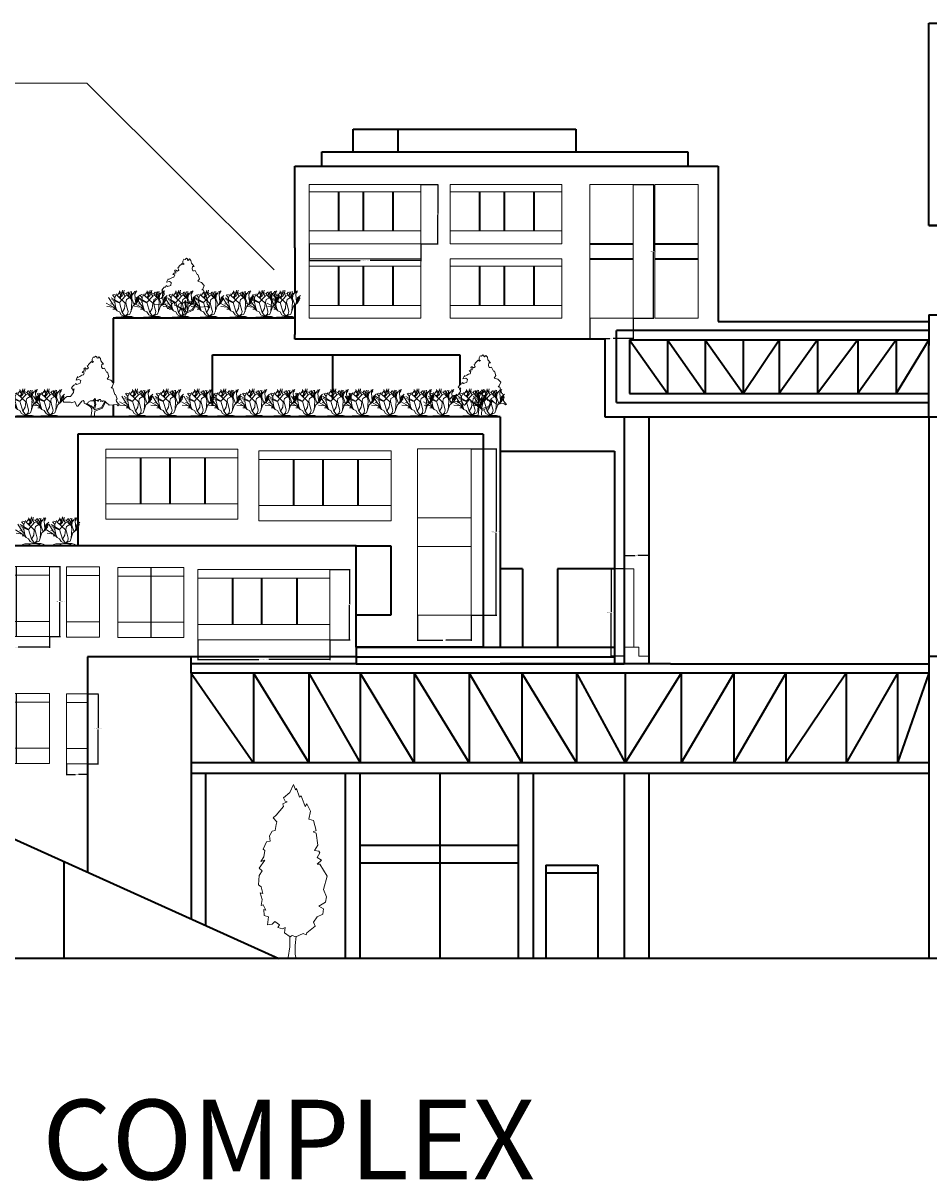
# Model space of a CAD drawing. Units: inches. Extents: x -1080 to 1950, y -1929 to 857.
# Tile 13 of 16: x 294 to 581, y -61 to 305. Entities that reach past the tile are written whole.
import ezdxf

# ---------------------------------------------------------------- set-up
doc = ezdxf.new("R2010")
doc.units = ezdxf.units.IN
doc.header["$MEASUREMENT"] = 0
for name, color, linetype, lineweight in [('A-ANNO-DIMS', 2, 'Continuous', 18), ('A-ANNO-SYMB', 2, 'Continuous', 18), ('A-ANNO-TEXT', 7, 'Continuous', 25), ('A-ELEV', 7, 'Continuous', 35), ('A-GLAZ', 4, 'Continuous', 18), ('L-PLNT', 82, 'Continuous', 13)]:
    doc.layers.add(name, color=color, linetype=linetype, lineweight=lineweight)
doc.styles.get("Standard").update_dxf_attribs({"font": 'arial.ttf'})
doc.dimstyles.get("Standard").update_dxf_attribs({"dimtxt": 0.18, "dimasz": 0.18, "dimexe": 0.18, "dimexo": 0.0625, "dimgap": 0.09, "dimtad": 0, "dimtih": 1, "dimtoh": 1, "dimdec": 4, "dimzin": 0, "dimdsep": 46, "dimtxsty": 'Standard', "dimcen": 0.09, "dimadec": 0, "dimazin": 0, "dimtfac": 1, "dimtdec": 4, "dimtofl": 0, "dimtmove": 0, "dimatfit": 3, "dimfxl": 1, "dimtolj": 1, "dimtzin": 0, "dimarcsym": 0})

# ---------------------------------------------------------------- blocks, each defined once
blk = doc.blocks.new('*U5')
blk.add_lwpolyline([(-2.754, 191.699), (-6.78, 182.851), (-13.682, 176.953), (-11.956, 173.266), (-9.656, 172.529), (-14.257, 170.317), (-13.682, 167.368), (-21.733, 157.783), (-25.184, 154.834), (-21.158, 150.41), (-21.733, 147.461), (-22.884, 140.825), (-26.334, 140.087), (-29.21, 134.926), (-28.635, 129.028), (-32.661, 128.291), (-36.111, 120.18), (-34.386, 118.706), (-35.536, 111.333), (-38.987, 106.171), (-34.386, 107.646), (-40.712, 98.798), (-37.261, 95.849), (-40.712, 90.688), (-41.287, 80.366), (-38.412, 78.154), (-36.686, 70.781), (-39.562, 71.518), (-37.261, 64.145), (-38.412, 57.509), (-36.111, 58.247), (-33.236, 52.348), (-35.536, 53.086), (-34.961, 46.45), (-30.36, 44.975), (-31.51, 36.128), (-26.334, 36.865), (-23.459, 39.814), (-18.283, 36.128), (-20.008, 33.178), (-14.832, 31.704), (-11.956, 33.178), (-12.531, 27.28), (-6.205, 22.856), (-3.905, 24.331), (0.121, 22.856), (8.173, 26.543), (11.624, 25.068), (12.199, 27.28), (21.4, 34.653), (19.675, 39.077), (23.701, 44.975), (30.027, 47.924), (30.602, 53.823), (25.426, 56.772), (32.903, 61.196), (34.053, 67.094), (30.602, 75.205), (34.628, 89.951), (26.576, 103.222), (23.701, 103.222), (28.302, 107.646), (23.701, 110.595), (26.576, 115.756), (25.426, 117.968), (20.825, 118.706), (24.276, 124.604), (22.551, 137.876), (19.1, 139.35), (22.551, 140.825), (19.675, 151.884), (14.499, 153.359), (16.224, 162.207), (12.199, 170.317), (10.473, 167.368), (5.872, 179.165), (4.147, 177.69), (0.696, 187.275), (-0.454, 185.8)], close=True)
for points in [[(-6.813, 23.669), (-6.813, 11.669), (-8.627, 0)], [(0.387, 23.669), (-0.576, 13.271), (-0.576, 3.686), (0, 0)]]:
    blk.add_lwpolyline(points)
blk = doc.blocks.new('*U2')
for points in [[(22.0124, 137.721), (18.5475, 141.5624), (15.5282, 138.2446), (13.8028, 139.3505), (13.3714, 142.1153), (11.2148, 143.2214), (8.1954, 140.4564), (4.7447, 141.0094), (2.1567, 136.0326), (2.1567, 131.6088), (5.6074, 129.9499), (3.0193, 128.2909), (0.4313, 130.5029), (-6.9015, 123.3141), (-6.9015, 121.6552), (-9.9208, 119.9963), (-9.0581, 118.3373), (-6.9015, 115.0195), (-10.7835, 112.2546), (-14.6656, 115.0195), (-16.8222, 114.4665), (-17.6849, 112.2546), (-14.6656, 111.7016), (-14.2342, 107.2778), (-17.6065, 107.8307), (-21.5669, 103.9599), (-17.2536, 103.4069), (-18.9789, 97.8771), (-22.8609, 97.3241), (-27.1743, 94.5593), (-32.3504, 91.7944), (-32.7817, 94.0063), (-36.6638, 85.7116), (-29.7624, 87.3705), (-25.449, 84.6056), (-26.743, 77.9699), (-34.507, 75.205), (-37.9578, 77.4169), (-39.2518, 74.099), (-42.2711, 73.5461), (-44.8592, 70.2282), (-47.8786, 66.3574), (-43.9965, 63.0395), (-41.4085, 64.6985), (-44.3346, 59.8898), (-42.2089, 60.1377), (-42.5159, 55.7849), (-49.6039, 46.4502), (-58.2307, 45.8972), (-62.1127, 43.6853), (-68.5828, 36.4966), (-65.9947, 32.0727), (-50.0352, 32.6257), (-47.0159, 30.4138), (-39.6831, 33.7317), (-34.507, 22.6721), (-32.3504, 22.6721), (-22.4296, 34.8376), (-19.4102, 36.4966), (-17.2536, 33.7317), (-17.2536, 29.8608), (-13.8028, 28.7549), (-9.0581, 28.7549), (-7.3328, 32.6257), (-1.7254, 35.3906), (3.8821, 35.9436), (6.4701, 38.1555), (6.9014, 38.7085), (8.1954, 41.4734), (9.9208, 40.3674), (11.2148, 35.9436), (14.2341, 37.6025), (15.0968, 36.4966), (15.9595, 33.7317), (18.9789, 38.7085), (21.9982, 38.7085), (23.2922, 36.4966), (21.9982, 34.2847), (25.4489, 35.3906), (26.743, 33.7317), (29.7623, 35.9436), (32.7817, 34.8376), (38.8204, 28.7549), (41.4084, 27.6489), (43.5651, 25.437), (61.6813, 27.0959), (65.132, 23.7781), (67.7201, 24.884), (60.8186, 33.7317), (60.3873, 37.0495), (62.544, 40.3674), (58.662, 50.874), (56.5053, 50.874), (52.1919, 66.3574), (47.8785, 66.9103), (50.4665, 69.1222), (53.9172, 77.9699), (47.0158, 85.1586), (38.3891, 87.9235), (42.2711, 94.0063)], [(42.2711, 94.0063), (38.8204, 104.5129), (36.6637, 104.5129), (32.3503, 113.9135), (29.7623, 113.3605), (26.743, 113.3605), (24.5862, 117.7844), (25.8802, 123.8671), (29.331, 123.8671), (22.8609, 131.6088), (21.9982, 137.6916)], [(-12.9401, 28.7549), (-2.588, 22.1191), (0.8626, 17.6953), (1.7253, 11.6125), (0, 0)], [(-9.9208, 28.2019), (0, 23.2251), (3.4507, 19.9072), (4.7447, 15.4834), (8.6267, 27.0959), (6.4701, 37.6025)], [(34.5071, 33.1787), (27.1743, 18.2483), (9.0581, 10.5066), (7.7641, 3.8708), (8.1954, 0)], [(8.1954, 40.3674), (11.2148, 27.6489), (8.1954, 13.8245), (24.5862, 19.9072), (32.7817, 34.2847)]]:
    blk.add_lwpolyline(points)
blk = doc.blocks.new('*U6')
for p, q in [((-377.952, 463.296), (-451.104, 487.68)), ((-426.72, 414.528), (-390.144, 499.872)), ((-377.952, 463.296), (-329.184, 524.256)), ((-316.7634, 502.285), (-327.6092, 559.9176)), ((-296.5958, 484.4034), (-316.7634, 502.285)), ((-286.512, 498.3226), (-307.4416, 538.0736)), ((-302.7934, 478.4344), (-270.256, 518.1854)), ((-290.3982, 464.5406), (-265.6078, 577.8246)), ((-268.7066, 458.5716), (-250.0884, 500.3038)), ((-207.264, 451.104), (-268.224, 548.64)), ((-240.792, 502.285), (-228.3968, 573.8368)), ((-182.88, 499.872), (-219.456, 512.064)), ((-207.264, 451.104), (-134.112, 487.68)), ((-182.88, 499.872), (-158.496, 536.448)), ((-121.92, 414.528), (-182.88, 499.872)), ((-129.1844, 450.6214), (-140.0302, 542.036)), ((-134.112, 487.68), (-97.536, 548.64)), ((-73.152, 329.184), (-109.728, 499.872)), ((-97.536, 426.72), (-24.384, 524.256)), ((-85.7758, 472.4908), (-73.3552, 548.005)), ((-73.152, 402.336), (-60.96, 512.064)), ((-12.9032, 555.9552), (-2.0574, 522.1732)), ((-5.1562, 486.3846), (2.5908, 542.036)), ((8.7884, 335.3562), (-5.1562, 486.3846)), ((-3.6068, 492.3536), (14.986, 518.1854)), ((-0.508, 508.254), (22.7584, 536.067)), ((1.0414, 526.1356), (35.1536, 559.9176)), ((2.5908, 542.036), (21.209, 555.9552)), ((-451.104, 219.456), (-601.0402, 303.8094)), ((-463.296, 280.416), (-552.577, 423.037)), ((-463.296, 280.416), (-512.064, 292.608)), ((-329.184, 316.992), (-499.872, 414.528)), ((-353.568, 316.992), (-487.68, 377.952)), ((-426.72, 414.528), (-475.488, 475.488)), ((-402.336, 207.264), (-463.296, 280.416)), ((-426.72, 316.992), (-451.104, 329.184)), ((-426.72, 316.992), (-426.72, 414.528)), ((-402.336, 207.264), (-426.72, 316.992)), ((-207.264, 304.8), (-377.952, 463.296)), ((-329.184, 316.992), (-353.568, 316.992)), ((-338.455, 424.7896), (-290.3982, 464.5406)), ((-329.184, 316.992), (-207.264, 451.104)), ((-268.224, 109.728), (-329.184, 316.992)), ((-305.8922, 396.9512), (-302.7934, 478.4344)), ((-304.3428, 426.7708), (-268.7066, 458.5716)), ((-219.456, 195.072), (-207.264, 304.8)), ((-195.072, 316.992), (-182.88, 377.952)), ((-170.688, 219.456), (-195.072, 316.992)), ((-182.88, 377.952), (-97.536, 426.72)), ((-85.7758, 389.001), (-129.1844, 452.6026)), ((-109.728, 73.152), (-48.768, 243.84)), ((-70.2564, 426.7708), (-85.7758, 472.4908)), ((-85.344, 134.112), (-73.152, 329.184)), ((-24.384, 268.224), (-73.152, 402.336)), ((-48.768, 243.84), (24.384, 304.8)), ((-12.192, 274.32), (8.7884, 335.3562)), ((8.7884, 335.3562), (33.6042, 412.8516)), ((24.384, 304.8), (36.576, 390.144)), ((24.384, 304.8), (73.152, 377.952)), ((33.6042, 412.8516), (92.5068, 464.5406)), ((36.576, 390.144), (73.152, 438.912)), ((48.768, 341.376), (60.96, 390.144)), ((60.96, 390.144), (85.344, 414.528)), ((-451.104, 219.456), (-587.4512, 234.2388)), ((-414.528, 182.88), (-463.296, 182.88)), ((-377.952, 146.304), (-451.104, 219.456)), ((-402.336, 12.192), (-451.104, 0)), ((-377.952, 146.304), (-402.336, 207.264)), ((-341.376, 12.192), (-402.336, 12.192)), ((-329.184, 121.92), (-377.952, 146.304)), ((-243.84, 24.384), (-341.376, 12.192)), ((-292.608, 60.96), (-329.184, 121.92)), ((-243.84, 24.384), (-329.184, 0)), ((-219.456, 24.384), (-292.608, 60.96)), ((-268.224, 109.728), (-219.456, 195.072)), ((-219.456, 48.768), (-268.224, 109.728)), ((-243.84, 24.384), (-195.072, 24.384)), ((-219.456, 24.384), (-109.728, 73.152)), ((-219.456, 24.384), (-158.496, 73.152)), ((-219.456, 24.384), (-219.456, 48.768)), ((-219.456, 24.384), (-73.152, 24.384)), ((-195.072, 24.384), (-158.496, 12.192)), ((-146.304, 134.112), (-170.688, 219.456)), ((-158.496, 73.152), (-146.304, 134.112)), ((-158.496, 12.192), (-85.344, 0)), ((-73.152, 24.384), (0, 0))]:
    blk.add_line(p, q)
blk = doc.blocks.new('*U4')
for points in [[(559.11496, 3498.1134), (471.1065, 3595.68496), (394.41628, 3511.41284), (350.59112, 3539.5027), (339.63356, 3609.72862), (284.85592, 3637.82356), (208.16316, 3567.59256), (120.51538, 3581.63876), (54.78018, 3455.22804), (54.78018, 3342.86352), (142.42796, 3300.72746), (76.69022, 3258.58886), (10.95502, 3314.77366), (-175.2981, 3132.17814), (-175.2981, 3090.04208), (-251.98832, 3047.90602), (-230.07574, 3005.76742), (-175.2981, 2921.4953), (-273.9009, 2851.26684), (-372.50624, 2921.4953), (-427.28388, 2907.4491), (-449.19646, 2851.26684), (-372.50624, 2837.22064), (-361.54868, 2724.85612), (-447.2051, 2738.89978), (-547.79926, 2640.58146), (-438.24144, 2626.53526), (-482.06406, 2486.07834), (-580.66686, 2472.03214), (-690.22722, 2401.80622), (-821.70016, 2331.57776), (-832.65518, 2387.76002), (-931.26052, 2177.07464), (-755.96496, 2219.2107), (-646.4046, 2148.98224), (-679.2722, 1980.43546), (-876.4778, 1910.207), (-964.12812, 1966.38926), (-996.99572, 1882.1146), (-1073.68594, 1868.07094), (-1139.42368, 1783.79628), (-1216.11644, 1685.47796), (-1117.5111, 1601.2033), (-1051.7759, 1643.3419), (-1126.09884, 1521.20092), (-1072.10606, 1527.49758), (-1079.90386, 1416.93646), (-1259.93906, 1179.83508), (-1479.05978, 1165.78888), (-1577.66258, 1109.60662), (-1742.00312, 927.01364), (-1676.26538, 814.64658), (-1270.89408, 828.69278), (-1194.20386, 772.51052), (-1007.95074, 856.78518), (-876.4778, 575.87134), (-821.70016, 575.87134), (-569.71184, 884.87504), (-493.01908, 927.01364), (-438.24144, 856.78518), (-438.24144, 758.46432), (-350.59112, 730.37446), (-230.07574, 730.37446), (-186.25312, 828.69278), (-43.82516, 898.92124), (98.60534, 912.96744), (164.34054, 969.1497), (175.29556, 983.1959), (208.16316, 1053.42436), (251.98832, 1025.33196), (284.85592, 912.96744), (361.54614, 955.1035), (383.45872, 927.01364), (405.3713, 856.78518), (482.06406, 983.1959), (558.75428, 983.1959), (591.62188, 927.01364), (558.75428, 870.83138), (646.40206, 898.92124), (679.2722, 856.78518), (755.96242, 912.96744), (832.65518, 884.87504), (986.03816, 730.37446), (1051.77336, 702.28206), (1106.55354, 646.0998), (1566.70502, 688.23586), (1654.3528, 603.96374), (1720.09054, 632.0536), (1544.79244, 856.78518), (1533.83742, 941.0573), (1588.6176, 1025.33196), (1490.0148, 1292.1996), (1435.23462, 1292.1996), (1325.67426, 1685.47796), (1216.1139, 1699.52162), (1281.8491, 1755.70388), (1369.49688, 1980.43546), (1194.20132, 2163.02844), (975.08314, 2233.2569), (1073.68594, 2387.76002)], [(1073.68594, 2387.76002), (986.03816, 2654.62766), (931.25798, 2654.62766), (821.69762, 2893.4029), (755.96242, 2879.3567), (679.2722, 2879.3567), (624.48948, 2991.72376), (657.35708, 3146.22434), (745.0074, 3146.22434), (580.66686, 3342.86352), (558.75428, 3497.36664)], [(-328.67854, 730.37446), (-65.7352, 561.82514), (21.91004, 449.46062), (43.82262, 294.9575), (0, 0)], [(-251.98832, 716.32826), (0, 589.91754), (87.64778, 505.64288), (120.51538, 393.27836), (219.11818, 688.23586), (164.34054, 955.1035)], [(876.48034, 842.73898), (690.22722, 463.50682), (230.07574, 266.86764), (197.20814, 98.31832), (208.16316, 0)], [(208.16316, 1025.33196), (284.85592, 702.28206), (208.16316, 351.1423), (624.48948, 505.64288), (832.65518, 870.83138)]]:
    blk.add_lwpolyline(points)
blk = doc.blocks.new('WIN-TYPE-B')
for p, q in [((10.5, 22.21), (0, 22.21)), ((0, 22.21), (0, 19.45)), ((20.91, 22.21), (10.41, 22.21)), ((10.41, 22.21), (10.41, 19.45)), ((10.5, 22.21), (10.5, 19.45)), ((20.91, 22.21), (20.91, 19.45)), ((0, 19.45), (0, 4.84)), ((0, 19.45), (10.5, 19.45)), ((10.41, 19.45), (10.41, 4.84)), ((10.41, 19.45), (20.91, 19.45)), ((10.5, 4.84), (10.5, 19.45)), ((20.91, 4.84), (20.91, 19.45)), ((0, 4.84), (10.5, 4.84)), ((0, 4.84), (0, 0)), ((10.41, 4.84), (20.91, 4.84)), ((10.41, 4.84), (10.41, 0)), ((10.5, 0), (10.5, 4.84)), ((20.91, 0), (20.91, 4.84)), ((0, 0), (10.5, 0)), ((10.41, 0), (20.91, 0))]:
    blk.add_line(p, q)
blk = doc.blocks.new('WIN-TYPE-E')
for p, q in [((10.5, 22.21), (0, 22.21)), ((0, 22.21), (0, 19.45)), ((10.5, 22.21), (10.5, 19.45)), ((0, 19.45), (0, 4.84)), ((0, 19.45), (10.5, 19.45)), ((10.5, 4.84), (10.5, 19.45)), ((0, 4.84), (10.5, 4.84)), ((0, 4.84), (0, 0)), ((10.5, 0), (10.5, 4.84)), ((0, 0), (10.5, 0))]:
    blk.add_line(p, q)
blk = doc.blocks.new('WIN-TYPE-G')
for p, q in [((0, 19.45), (0, 22.21)), ((0, 22.21), (41.85, 22.21)), ((41.85, 22.21), (41.85, 19.45)), ((0, 19.45), (0, 4.84)), ((41.85, 19.45), (0, 19.45)), ((41.85, 4.84), (41.85, 19.45)), ((0, 4.84), (41.85, 4.84)), ((0, 4.84), (0, 0)), ((41.85, 0), (41.85, 4.84)), ((0, 0), (41.85, 0))]:
    blk.add_line(p, q)
blk = doc.blocks.new('WIN-TYPE-H')
for p, q in [((0, 16.47), (0, 18.8)), ((0, 18.8), (35.42, 18.8)), ((35.42, 18.8), (35.42, 16.47)), ((0, 16.47), (0, 4.09)), ((35.42, 16.47), (0, 16.47)), ((35.42, 4.09), (35.42, 16.47)), ((0, 4.09), (35.42, 4.09)), ((0, 4.09), (0, 0)), ((35.42, 0), (35.42, 4.09)), ((0, 0), (35.42, 0))]:
    blk.add_line(p, q)
blk = doc.blocks.new('WIN-TYPE-N')
for p, q in [((0, 52.66), (17.07, 52.66)), ((0, 30.88), (0, 52.66)), ((17.07, 52.66), (17.07, 30.88)), ((17.07, 30.88), (0, 30.88)), ((0, 30.88), (0, 21.78)), ((17.07, 30.88), (17.07, 21.78)), ((0, 21.78), (17.07, 21.78)), ((0, 0), (0, 21.78)), ((17.07, 21.78), (17.07, 0)), ((17.07, 0), (0, 0))]:
    blk.add_line(p, q)
blk = doc.blocks.new('PANEL-A')
for p, q in [((0, 42.42), (0, 0)), ((13.76, 42.42), (0, 42.42)), ((13.76, 0), (13.76, 42.42)), ((0, 0), (13.76, 0))]:
    blk.add_line(p, q)
blk = doc.blocks.new('WIN-TYPE-R')
for p, q in [((6.66, 22.21), (0, 22.21)), ((0, 22.21), (0, 19.45)), ((0, 19.45), (0, 4.84)), ((0, 19.45), (6.66, 19.45)), ((0, 4.84), (6.66, 4.84)), ((0, 4.84), (0, 0)), ((0, 0), (6.66, 0))]:
    blk.add_line(p, q)
blk = doc.blocks.new('WIN-TYPE-S')
for p, q in [((0, 27.66), (3.06, 27.66)), ((3.06, 27.66), (3.06, 2.78)), ((3.06, 2.78), (0, 2.78)), ((3.06, 2.78), (4.6, 2.78)), ((4.6, 2.78), (4.6, 0)), ((4.6, 0), (7.75, 0))]:
    blk.add_line(p, q)
blk = doc.blocks.new('*D37')
at = {"layer": 'A-ANNO-DIMS', "color": 0, "lineweight": -2, "transparency": 16777216}
for p, q in [((302.32, 133.16), (305.76, 133.16)), ((305.58, 132.98), (305.58, 122.24)), ((305.58, 111.13), (305.58, 121.87)), ((302.32, 110.95), (305.76, 110.95))]:
    blk.add_line(p, q, dxfattribs=at)
at = {"layer": 'A-ANNO-DIMS', "color": 0, "transparency": 16777216}
for points in [[(305.55, 132.98), (305.61, 132.98), (305.58, 133.16)], [(305.55, 111.13), (305.61, 111.13), (305.58, 110.95)]]:
    blk.add_solid(points, dxfattribs=at)
at = {"layer": 'Defpoints', "color": 0, "transparency": 16777216}
for p in [(302.25, 133.16), (305.58, 133.16), (302.25, 110.95)]:
    blk.add_point(p, dxfattribs=at)
at = {"layer": 'A-ANNO-DIMS', "color": 0, "transparency": 16777216, "insert": (305.58, 122.05), "char_height": 0.18, "attachment_point": 5}
blk.add_mtext('\\A1;WINDOW TYPE B 22 TYP.', dxfattribs=at)
blk = doc.blocks.new('*D38')
at = {"layer": 'A-ANNO-DIMS', "color": 0, "lineweight": -2, "transparency": 16777216}
for p, q in [((281.34, 110.89), (281.34, 107.44)), ((302.25, 110.89), (302.25, 107.44)), ((281.52, 107.62), (291.27, 107.62)), ((302.07, 107.62), (292.33, 107.62))]:
    blk.add_line(p, q, dxfattribs=at)
at = {"layer": 'A-ANNO-DIMS', "color": 0, "transparency": 16777216}
for points in [[(281.52, 107.65), (281.52, 107.59), (281.34, 107.62)], [(302.07, 107.65), (302.07, 107.59), (302.25, 107.62)]]:
    blk.add_solid(points, dxfattribs=at)
at = {"layer": 'Defpoints', "color": 0, "transparency": 16777216}
for p in [(281.34, 110.95), (302.25, 110.95), (302.25, 107.62)]:
    blk.add_point(p, dxfattribs=at)
at = {"layer": 'A-ANNO-DIMS', "color": 0, "transparency": 16777216, "insert": (291.8, 107.62), "char_height": 0.18, "attachment_point": 5}
blk.add_mtext('\\A1;21 TYP.', dxfattribs=at)
blk = doc.blocks.new('*D47')
at = {"layer": 'A-ANNO-DIMS', "color": 0, "lineweight": -2, "transparency": 16777216}
for p, q in [((349.28, 109.92), (349.28, 103.52)), ((391.12, 109.92), (391.12, 103.52)), ((349.46, 103.7), (368.59, 103.7)), ((390.94, 103.7), (371.82, 103.7))]:
    blk.add_line(p, q, dxfattribs=at)
at = {"layer": 'A-ANNO-DIMS', "color": 0, "transparency": 16777216}
for points in [[(349.46, 103.73), (349.46, 103.67), (349.28, 103.7)], [(390.94, 103.73), (390.94, 103.67), (391.12, 103.7)]]:
    blk.add_solid(points, dxfattribs=at)
at = {"layer": 'Defpoints', "color": 0, "transparency": 16777216}
for p in [(349.28, 109.98), (391.12, 109.98), (391.12, 103.7)]:
    blk.add_point(p, dxfattribs=at)
at = {"layer": 'A-ANNO-DIMS', "color": 0, "transparency": 16777216, "insert": (370.2, 103.7), "char_height": 0.18, "attachment_point": 5}
blk.add_mtext('\\A1;WINDOW TYPE G 42 TYP.', dxfattribs=at)
blk = doc.blocks.new('*D48')
at = {"layer": 'A-ANNO-DIMS', "color": 0, "lineweight": -2, "transparency": 16777216}
for p, q in [((391.19, 132.19), (397.58, 132.19)), ((397.4, 132.01), (397.4, 121.27)), ((397.4, 110.16), (397.4, 120.9)), ((391.19, 109.98), (397.58, 109.98))]:
    blk.add_line(p, q, dxfattribs=at)
at = {"layer": 'A-ANNO-DIMS', "color": 0, "transparency": 16777216}
for points in [[(397.37, 132.01), (397.43, 132.01), (397.4, 132.19)], [(397.37, 110.16), (397.43, 110.16), (397.4, 109.98)]]:
    blk.add_solid(points, dxfattribs=at)
at = {"layer": 'Defpoints', "color": 0, "transparency": 16777216}
for p in [(391.12, 132.19), (397.4, 132.19), (391.12, 109.98)]:
    blk.add_point(p, dxfattribs=at)
at = {"layer": 'A-ANNO-DIMS', "color": 0, "transparency": 16777216, "insert": (397.4, 121.08), "char_height": 0.18, "attachment_point": 5}
blk.add_mtext('\\A1;22 TYP.', dxfattribs=at)
blk = doc.blocks.new('*D49')
at = {"layer": 'A-ANNO-DIMS', "color": 0, "lineweight": -2, "transparency": 16777216}
for p, q in [((384.59, 235.36), (384.59, 229.93)), ((420.01, 235.36), (420.01, 229.93)), ((384.77, 230.11), (400.7, 230.11)), ((419.83, 230.11), (403.91, 230.11))]:
    blk.add_line(p, q, dxfattribs=at)
at = {"layer": 'A-ANNO-DIMS', "color": 0, "transparency": 16777216}
for points in [[(384.77, 230.14), (384.77, 230.08), (384.59, 230.11)], [(419.83, 230.14), (419.83, 230.08), (420.01, 230.11)]]:
    blk.add_solid(points, dxfattribs=at)
at = {"layer": 'Defpoints', "color": 0, "transparency": 16777216}
for p in [(384.59, 235.42), (420.01, 235.42), (420.01, 230.11)]:
    blk.add_point(p, dxfattribs=at)
at = {"layer": 'A-ANNO-DIMS', "color": 0, "transparency": 16777216, "insert": (402.3, 230.11), "char_height": 0.18, "attachment_point": 5}
blk.add_mtext('\\A1;WINDOW TYPE H 35 TYP.', dxfattribs=at)
blk = doc.blocks.new('*D50')
at = {"layer": 'A-ANNO-DIMS', "color": 0, "lineweight": -2, "transparency": 16777216}
for p, q in [((420.08, 254.22), (425.51, 254.22)), ((425.33, 254.04), (425.33, 245)), ((425.33, 235.6), (425.33, 244.64)), ((420.08, 235.42), (425.51, 235.42))]:
    blk.add_line(p, q, dxfattribs=at)
at = {"layer": 'A-ANNO-DIMS', "color": 0, "transparency": 16777216}
for points in [[(425.3, 254.04), (425.36, 254.04), (425.33, 254.22)], [(425.3, 235.6), (425.36, 235.6), (425.33, 235.42)]]:
    blk.add_solid(points, dxfattribs=at)
at = {"layer": 'Defpoints', "color": 0, "transparency": 16777216}
for p in [(420.01, 254.22), (425.33, 254.22), (420.01, 235.42)]:
    blk.add_point(p, dxfattribs=at)
at = {"layer": 'A-ANNO-DIMS', "color": 0, "transparency": 16777216, "insert": (425.33, 244.82), "char_height": 0.18, "attachment_point": 5}
blk.add_mtext('\\A1;19 TYP.', dxfattribs=at)
blk = doc.blocks.new('*D59')
at = {"layer": 'A-ANNO-DIMS', "color": 0, "lineweight": -2, "transparency": 16777216}
for p, q in [((436.01, 170.39), (444.03, 170.39)), ((443.85, 170.21), (443.85, 144.25)), ((443.85, 117.91), (443.85, 143.88)), ((436.01, 117.73), (444.03, 117.73))]:
    blk.add_line(p, q, dxfattribs=at)
at = {"layer": 'A-ANNO-DIMS', "color": 0, "transparency": 16777216}
for points in [[(443.82, 170.21), (443.88, 170.21), (443.85, 170.39)], [(443.82, 117.91), (443.88, 117.91), (443.85, 117.73)]]:
    blk.add_solid(points, dxfattribs=at)
at = {"layer": 'Defpoints', "color": 0, "transparency": 16777216}
for p in [(435.95, 170.39), (443.85, 170.39), (435.95, 117.73)]:
    blk.add_point(p, dxfattribs=at)
at = {"layer": 'A-ANNO-DIMS', "color": 0, "transparency": 16777216, "insert": (443.85, 144.06), "char_height": 0.18, "attachment_point": 5}
blk.add_mtext('\\A1;WINDOW TYPE N 53 TYP.', dxfattribs=at)
blk = doc.blocks.new('*D60')
at = {"layer": 'A-ANNO-DIMS', "color": 0, "lineweight": -2, "transparency": 16777216}
for p, q in [((418.88, 117.67), (418.88, 109.65)), ((435.95, 117.67), (435.95, 109.65)), ((419.06, 109.83), (426.89, 109.83)), ((435.77, 109.83), (427.93, 109.83))]:
    blk.add_line(p, q, dxfattribs=at)
at = {"layer": 'A-ANNO-DIMS', "color": 0, "transparency": 16777216}
for points in [[(419.06, 109.86), (419.06, 109.8), (418.88, 109.83)], [(435.77, 109.86), (435.77, 109.8), (435.95, 109.83)]]:
    blk.add_solid(points, dxfattribs=at)
at = {"layer": 'Defpoints', "color": 0, "transparency": 16777216}
for p in [(418.88, 117.73), (435.95, 117.73), (435.95, 109.83)]:
    blk.add_point(p, dxfattribs=at)
at = {"layer": 'A-ANNO-DIMS', "color": 0, "transparency": 16777216, "insert": (427.41, 109.83), "char_height": 0.18, "attachment_point": 5}
blk.add_mtext('\\A1;17 TYP.', dxfattribs=at)
blk = doc.blocks.new('*D65')
at = {"layer": 'A-ANNO-DIMS', "color": 0, "lineweight": -2, "transparency": 16777216}
for p, q in [((314.38, 92.83), (317.83, 92.83)), ((317.65, 92.65), (317.65, 81.91)), ((317.65, 70.8), (317.65, 81.54)), ((314.38, 70.62), (317.83, 70.62))]:
    blk.add_line(p, q, dxfattribs=at)
at = {"layer": 'A-ANNO-DIMS', "color": 0, "transparency": 16777216}
for points in [[(317.62, 92.65), (317.68, 92.65), (317.65, 92.83)], [(317.62, 70.8), (317.68, 70.8), (317.65, 70.62)]]:
    blk.add_solid(points, dxfattribs=at)
at = {"layer": 'Defpoints', "color": 0, "transparency": 16777216}
for p in [(314.32, 92.83), (317.65, 92.83), (314.32, 70.62)]:
    blk.add_point(p, dxfattribs=at)
at = {"layer": 'A-ANNO-DIMS', "color": 0, "transparency": 16777216, "insert": (317.65, 81.73), "char_height": 0.18, "attachment_point": 5}
blk.add_mtext('\\A1;WINDOW TYPE R 22 TYP.', dxfattribs=at)
blk = doc.blocks.new('*D66')
at = {"layer": 'A-ANNO-DIMS', "color": 0, "lineweight": -2, "transparency": 16777216}
for p, q in [((307.66, 70.56), (307.66, 67.11)), ((314.32, 70.56), (314.32, 67.11)), ((307.84, 67.29), (310.53, 67.29)), ((314.14, 67.29), (311.45, 67.29))]:
    blk.add_line(p, q, dxfattribs=at)
at = {"layer": 'A-ANNO-DIMS', "color": 0, "transparency": 16777216}
for points in [[(307.84, 67.32), (307.84, 67.26), (307.66, 67.29)], [(314.14, 67.32), (314.14, 67.26), (314.32, 67.29)]]:
    blk.add_solid(points, dxfattribs=at)
at = {"layer": 'Defpoints', "color": 0, "transparency": 16777216}
for p in [(307.66, 70.62), (314.32, 70.62), (314.32, 67.29)]:
    blk.add_point(p, dxfattribs=at)
at = {"layer": 'A-ANNO-DIMS', "color": 0, "transparency": 16777216, "insert": (310.99, 67.29), "char_height": 0.18, "attachment_point": 5}
blk.add_mtext('\\A1;7 TYP.', dxfattribs=at)
blk = doc.blocks.new('*D67')
at = {"layer": 'A-ANNO-DIMS', "color": 0, "lineweight": -2, "transparency": 16777216}
for p, q in [((484.36, 132.47), (480.1, 132.47)), ((480.28, 132.29), (480.28, 118.82)), ((480.28, 104.99), (480.28, 118.45)), ((484.36, 104.81), (480.1, 104.81))]:
    blk.add_line(p, q, dxfattribs=at)
at = {"layer": 'A-ANNO-DIMS', "color": 0, "transparency": 16777216}
for points in [[(480.25, 132.29), (480.31, 132.29), (480.28, 132.47)], [(480.25, 104.99), (480.31, 104.99), (480.28, 104.81)]]:
    blk.add_solid(points, dxfattribs=at)
at = {"layer": 'Defpoints', "color": 0, "transparency": 16777216}
for p in [(480.28, 132.47), (484.43, 132.47), (484.43, 104.81)]:
    blk.add_point(p, dxfattribs=at)
at = {"layer": 'A-ANNO-DIMS', "color": 0, "transparency": 16777216, "insert": (480.28, 118.64), "char_height": 0.18, "attachment_point": 5}
blk.add_mtext('\\A1;WINDOW TYPE S 28 TYP.', dxfattribs=at)
blk = doc.blocks.new('*D68')
at = {"layer": 'A-ANNO-DIMS', "color": 0, "lineweight": -2, "transparency": 16777216}
for p, q in [((484.43, 132.53), (484.43, 136.79)), ((484.61, 136.61), (487.85, 136.61)), ((492, 136.61), (488.76, 136.61)), ((492.18, 132.53), (492.18, 136.79))]:
    blk.add_line(p, q, dxfattribs=at)
at = {"layer": 'A-ANNO-DIMS', "color": 0, "transparency": 16777216}
for points in [[(484.61, 136.64), (484.61, 136.58), (484.43, 136.61)], [(492, 136.64), (492, 136.58), (492.18, 136.61)]]:
    blk.add_solid(points, dxfattribs=at)
at = {"layer": 'Defpoints', "color": 0, "transparency": 16777216}
for p in [(492.18, 136.61), (484.43, 132.47), (492.18, 132.47)]:
    blk.add_point(p, dxfattribs=at)
at = {"layer": 'A-ANNO-DIMS', "color": 0, "transparency": 16777216, "insert": (488.3, 136.61), "char_height": 0.18, "attachment_point": 5}
blk.add_mtext('\\A1;8 TYP.', dxfattribs=at)
blk = doc.blocks.new('*D71')
at = {"layer": 'A-ANNO-DIMS', "color": 0, "lineweight": -2, "transparency": 16777216}
for p, q in [((487.36, 254.22), (493.84, 254.22)), ((493.66, 254.04), (493.66, 233.19)), ((493.66, 211.98), (493.66, 232.83)), ((487.36, 211.8), (493.84, 211.8))]:
    blk.add_line(p, q, dxfattribs=at)
at = {"layer": 'A-ANNO-DIMS', "color": 0, "transparency": 16777216}
for points in [[(493.63, 254.04), (493.69, 254.04), (493.66, 254.22)], [(493.63, 211.98), (493.69, 211.98), (493.66, 211.8)]]:
    blk.add_solid(points, dxfattribs=at)
at = {"layer": 'Defpoints', "color": 0, "transparency": 16777216}
for p in [(487.3, 254.22), (493.66, 254.22), (487.3, 211.8)]:
    blk.add_point(p, dxfattribs=at)
at = {"layer": 'A-ANNO-DIMS', "color": 0, "transparency": 16777216, "insert": (493.66, 233.01), "char_height": 0.18, "attachment_point": 5}
blk.add_mtext('\\A1;PANEL A 42 TYP.', dxfattribs=at)
blk = doc.blocks.new('*D72')
at = {"layer": 'A-ANNO-DIMS', "color": 0, "lineweight": -2, "transparency": 16777216}
for p, q in [((473.54, 211.74), (473.54, 205.26)), ((487.3, 211.74), (487.3, 205.26)), ((473.72, 205.44), (479.9, 205.44)), ((487.12, 205.44), (480.94, 205.44))]:
    blk.add_line(p, q, dxfattribs=at)
at = {"layer": 'A-ANNO-DIMS', "color": 0, "transparency": 16777216}
for points in [[(473.72, 205.47), (473.72, 205.41), (473.54, 205.44)], [(487.12, 205.47), (487.12, 205.41), (487.3, 205.44)]]:
    blk.add_solid(points, dxfattribs=at)
at = {"layer": 'Defpoints', "color": 0, "transparency": 16777216}
for p in [(473.54, 211.8), (487.3, 211.8), (487.3, 205.44)]:
    blk.add_point(p, dxfattribs=at)
at = {"layer": 'A-ANNO-DIMS', "color": 0, "transparency": 16777216, "insert": (480.42, 205.44), "char_height": 0.18, "attachment_point": 5}
blk.add_mtext('\\A1;14 TYP.', dxfattribs=at)

msp = doc.modelspace()

# ---------------------------------------------------------------- linework, layer by layer
at = {"layer": 'A-ANNO-SYMB'}
for q in [(282.36, 286.23), (373.52, 227.18)]:
    msp.add_line((314.15, 286.23), q, dxfattribs=at)
at = {"layer": 'A-ELEV'}
for p, q in [((580.98, 305.29), (695.2, 305.29)), ((580.98, 241.18), (580.98, 305.29)), ((398.48, 269.6), (398.48, 271.66)), ((398.48, 271.66), (469.06, 271.66)), ((412.81, 264.54), (412.81, 271.66)), ((469.06, 271.66), (469.06, 264.54)), ((398.48, 264.54), (398.48, 269.6)), ((388.54, 260.04), (388.54, 264.54)), ((388.54, 264.54), (504.61, 264.54)), ((504.61, 264.54), (504.61, 260.04)), ((379.98, 250.46), (379.98, 260.04)), ((379.98, 260.04), (509.7, 260.04)), ((509.7, 260.04), (514.2, 260.04)), ((514.2, 260.04), (514.2, 210.83)), ((379.98, 234.12), (379.98, 250.46)), ((393.87, 251.89), (393.87, 239.51)), ((401.72, 251.89), (401.72, 239.51)), ((411.12, 251.89), (411.12, 239.51)), ((438.56, 251.89), (438.56, 239.51)), ((446.4, 251.89), (446.4, 239.51)), ((455.81, 251.89), (455.81, 239.51)), ((592.18, 241.18), (580.98, 241.18)), ((580.98, 241.18), (695.2, 241.18)), ((473.54, 235.42), (487.3, 235.42)), ((494.09, 235.42), (507.85, 235.42)), ((379.98, 234.12), (379.98, 219.88)), ((393.87, 228.27), (393.87, 215.89)), ((401.72, 228.27), (401.72, 215.89)), ((411.12, 228.27), (411.12, 215.89)), ((438.56, 228.27), (438.56, 215.89)), ((446.4, 228.27), (446.4, 215.89)), ((455.81, 228.27), (455.81, 215.89)), ((473.54, 230.6), (487.3, 230.6)), ((494.09, 230.6), (507.85, 230.6)), ((379.98, 216.14), (379.98, 206.68)), ((580.98, 212.94), (580.98, 203.15)), ((580.98, 212.94), (695.2, 212.94)), ((379.98, 211.8), (322.42, 211.8)), ((322.42, 211.8), (322.42, 191.39)), ((514.2, 210.83), (580.98, 210.83)), ((379.98, 205.21), (379.98, 206.68)), ((580.98, 207.88), (481.95, 207.88)), ((481.95, 185.16), (481.95, 207.88)), ((478.29, 205.21), (379.98, 205.21)), ((478.29, 205.21), (478.29, 185.16)), ((486.15, 204.96), (580.98, 204.96)), ((486.15, 204.96), (486.15, 188.02)), ((486.15, 204.96), (498.15, 188.02)), ((498.15, 204.96), (498.15, 188.02)), ((498.15, 204.96), (510.1, 188.02)), ((510.1, 204.96), (510.1, 188.02)), ((510.1, 204.96), (522.17, 188.02)), ((522.17, 204.96), (522.17, 188.02)), ((522.17, 188.02), (533.52, 204.96)), ((533.52, 204.96), (533.52, 188.02)), ((545.71, 204.96), (533.52, 188.02)), ((545.71, 204.96), (545.71, 188.02)), ((558.5, 204.96), (545.71, 188.02)), ((558.5, 204.96), (558.5, 188.02)), ((570.57, 204.96), (558.5, 188.02)), ((570.57, 204.96), (570.57, 188.02)), ((580.98, 204.96), (570.57, 188.02)), ((580.98, 180.63), (580.98, 203.15)), ((353.96, 187.18), (353.96, 200.27)), ((353.96, 200.27), (432.33, 200.27)), ((391.97, 200.27), (391.97, 186.07)), ((432.33, 200.27), (432.33, 190.71)), ((580.98, 183.28), (580.98, 200.23)), ((486.15, 188.02), (580.98, 188.02)), ((322.42, 184.41), (322.42, 180.63)), ((353.96, 184.1), (353.96, 185.92)), ((478.29, 185.16), (478.29, 180.63)), ((481.95, 185.16), (580.98, 185.16)), ((445.1, 180.63), (264.78, 180.63)), ((391.97, 180.95), (391.97, 180.63)), ((432.51, 180.68), (432.51, 180.63)), ((445.1, 180.63), (445.1, 107.59)), ((478.29, 180.63), (695.2, 180.63)), ((484.43, 180.63), (484.43, 102.28)), ((492.18, 180.63), (492.18, 102.28)), ((580.98, 180.63), (580.98, 104.79)), ((439.77, 175.14), (311.23, 175.14)), ((311.23, 175.14), (311.23, 146.63)), ((439.77, 175.14), (439.77, 107.59)), ((445.1, 169.72), (481.39, 169.72)), ((481.39, 169.72), (481.39, 102.28)), ((331.1, 167.62), (331.1, 153)), ((340.37, 167.62), (340.37, 153)), ((351.48, 167.62), (351.48, 153)), ((379.62, 167.07), (379.62, 152.45)), ((388.89, 167.07), (388.89, 152.45)), ((400, 167.07), (400, 152.45)), ((311.23, 145.47), (311.23, 139.7)), ((311.23, 139.7), (27.33, 139.7)), ((399.5, 139.7), (311.23, 139.7)), ((399.5, 107.59), (399.5, 139.7)), ((399.5, 139.7), (410.5, 139.7)), ((410.5, 139.7), (410.5, 117.73)), ((452.21, 132.47), (445.1, 132.47)), ((452.21, 132.47), (452.21, 107.59)), ((481.39, 132.47), (463.32, 132.47)), ((463.32, 132.47), (463.32, 107.59)), ((360.24, 129.43), (360.24, 114.82)), ((369.51, 129.43), (369.51, 114.82)), ((380.62, 129.43), (380.62, 114.82)), ((410.5, 117.73), (399.5, 117.73)), ((439.77, 107.59), (399.5, 107.59)), ((399.5, 107.59), (399.5, 102.28)), ((399.5, 107.59), (481.39, 107.59)), ((399.5, 104.57), (314.32, 104.57)), ((314.32, 104.57), (314.32, 102.28)), ((347.2, 102.28), (347.2, 104.57)), ((399.5, 104.57), (481.39, 104.57)), ((580.98, 104.79), (695.2, 104.79)), ((580.98, 104.79), (580.98, 65.68)), ((314.32, 102.28), (314.32, 36.38)), ((399.5, 102.28), (347.2, 102.28)), ((347.2, 99.4), (347.2, 102.28)), ((399.5, 99.4), (347.2, 99.4)), ((347.2, 99.4), (347.2, 25.36)), ((347.2, 99.4), (366.88, 70.95)), ((366.88, 99.4), (366.88, 70.95)), ((366.88, 99.4), (384.43, 70.95)), ((384.43, 99.4), (384.43, 70.95)), ((384.43, 99.4), (400.7, 70.95)), ((399.5, 102.28), (484.43, 102.28)), ((495.98, 99.4), (399.5, 99.4)), ((400.7, 99.4), (400.7, 70.95)), ((400.7, 99.4), (417.81, 70.95)), ((417.81, 99.4), (417.81, 70.95)), ((417.81, 99.4), (435.24, 70.95)), ((435.24, 99.4), (435.24, 70.95)), ((435.24, 99.4), (451.98, 70.95)), ((499.06, 102.28), (445.1, 102.28)), ((451.98, 99.4), (451.98, 70.95)), ((451.98, 99.4), (469.32, 70.95)), ((469.32, 99.4), (469.32, 70.95)), ((469.32, 99.4), (484.68, 70.95)), ((484.68, 99.4), (484.68, 70.95)), ((502.48, 99.4), (484.68, 70.95)), ((580.98, 99.4), (495.98, 99.4)), ((499.06, 102.28), (580.98, 102.28)), ((502.48, 99.4), (502.48, 70.95)), ((519.22, 99.4), (502.48, 70.95)), ((519.22, 99.4), (519.22, 70.95)), ((535.61, 99.4), (519.22, 70.95)), ((535.61, 99.4), (535.61, 70.95)), ((554.76, 99.4), (535.61, 70.95)), ((554.76, 99.4), (554.76, 70.95)), ((571.04, 99.4), (554.76, 70.95)), ((571.04, 99.4), (571.04, 70.95)), ((580.98, 99.4), (571.04, 70.95)), ((221.9, 78.07), (374.96, 9.02)), ((499.06, 70.95), (347.2, 70.95)), ((580.98, 70.95), (499.06, 70.95)), ((510.1, 67.56), (347.2, 67.56)), ((351.73, 67.56), (351.73, 19.5)), ((395.95, 67.56), (395.95, 9.02)), ((400.61, 67.56), (400.61, 9.02)), ((426.02, 67.56), (426.02, 9.02)), ((450.86, 67.56), (450.86, 9.02)), ((455.52, 67.56), (455.52, 9.02)), ((484.43, 67.56), (484.43, 9.02)), ((492.18, 67.56), (492.18, 9.02)), ((580.98, 67.56), (510.1, 67.56)), ((580.98, 65.68), (580.98, 9.02)), ((400.61, 44.86), (450.86, 44.86)), ((306.83, 39.76), (306.83, 9.02)), ((400.61, 39.31), (450.86, 39.31)), ((459.6, 38.54), (476.06, 38.54)), ((459.6, 38.54), (459.6, 9.02)), ((476.06, 38.54), (476.06, 9.02)), ((459.6, 36.1), (476.06, 36.1)), ((347.2, 25.36), (347.2, 21.54)), ((709.45, 9.02), (-148.56, 9.02))]:
    msp.add_line(p, q, dxfattribs=at)

# ---------------------------------------------------------------- block references
at = {"layer": 'A-GLAZ'}
for name, p in [('WIN-TYPE-H', (384.59, 235.42)), ('WIN-TYPE-H', (429.28, 235.42)), ('PANEL-A', (473.54, 211.8)), ('PANEL-A', (494.09, 211.8)), ('WIN-TYPE-H', (384.59, 211.8)), ('WIN-TYPE-H', (429.28, 211.8)), ('WIN-TYPE-G', (320.14, 148.16)), ('WIN-TYPE-G', (368.66, 147.62)), ('WIN-TYPE-N', (418.88, 117.73)), ('WIN-TYPE-B', (281.34, 110.95)), ('WIN-TYPE-E', (307.66, 110.83)), ('WIN-TYPE-B', (323.96, 110.64)), ('WIN-TYPE-G', (349.28, 109.98)), ('WIN-TYPE-S', (484.43, 104.81)), ('WIN-TYPE-B', (281.34, 70.74)), ('WIN-TYPE-R', (307.66, 70.62))]:
    msp.add_blockref(name, p, dxfattribs=at)
at = {"layer": 'L-PLNT'}
for name, p, xscale, yscale, zscale in [('*U2', (344.22, 211.96), 0.1315554675521508, 0.1315554675521508, 0.1315554675521508), ('*U6', (329.43, 211.95), 0.0152219259934872, 0.0152219259934872, 0.0152219259934872), ('*U6', (338.17, 211.95), 0.0152219259934872, 0.0152219259934872, 0.0152219259934872), ('*U6', (347.28, 211.95), 0.0152219259934872, 0.0152219259934872, 0.0152219259934872), ('*U6', (356.14, 211.95), 0.0152219259934872, 0.0152219259934872, 0.0152219259934872), ('*U6', (365.54, 211.95), 0.0152219259934872, 0.0152219259934872, 0.0152219259934872), ('*U6', (373.75, 211.95), 0.0152219259934872, 0.0152219259934872, 0.0152219259934872), ('*U6', (380.38, 211.95), 0.0152219259934872, 0.0152219259934872, 0.0152219259934872), ('*U2', (315.5, 180.96), 0.1315554675521508, 0.1315554675521508, 0.1315554675521508), ('*U4', (438.13, 181.23), 0.0052143573184964, 0.0052143573184964, 0.0052143573184964), ('*U6', (297.89, 180.68), 0.0152219259934872, 0.0152219259934872, 0.0152219259934872), ('*U6', (305.63, 180.68), 0.0152219259934872, 0.0152219259934872, 0.0152219259934872), ('*U6', (333.59, 180.68), 0.0152219259934872, 0.0152219259934872, 0.0152219259934872), ('*U6', (343.36, 180.68), 0.0152219259934872, 0.0152219259934872, 0.0152219259934872), ('*U6', (353.21, 180.68), 0.0152219259934872, 0.0152219259934872, 0.0152219259934872), ('*U6', (361.6, 180.68), 0.0152219259934872, 0.0152219259934872, 0.0152219259934872), ('*U6', (370.64, 180.68), 0.0152219259934872, 0.0152219259934872, 0.0152219259934872), ('*U6', (379.53, 180.68), 0.0152219259934872, 0.0152219259934872, 0.0152219259934872), ('*U6', (387.43, 180.68), 0.0152219259934872, 0.0152219259934872, 0.0152219259934872), ('*U6', (396.47, 180.68), 0.0152219259934872, 0.0152219259934872, 0.0152219259934872), ('*U6', (404.37, 180.68), 0.0152219259934872, 0.0152219259934872, 0.0152219259934872), ('*U6', (413.27, 180.68), 0.0152219259934872, 0.0152219259934872, 0.0152219259934872), ('*U6', (422.86, 180.68), 0.0152219259934872, 0.0152219259934872, 0.0152219259934872), ('*U6', (429.92, 180.68), 0.0152219259934872, 0.0152219259934872, 0.0152219259934872), ('*U6', (439.38, 180.68), 0.0152219259934872, 0.0152219259934872, 0.0152219259934872), ('*U6', (445.07, 180.68), 0.0152219259934872, 0.0152219259934872, 0.0152219259934872), ('*U6', (300.62, 140.11), 0.0152219259934872, 0.0152219259934872, 0.0152219259934872), ('*U6', (310.45, 140.11), 0.0152219259934872, 0.0152219259934872, 0.0152219259934872), ('*U5', (380.35, 9.33), 0.2857357741909547, 0.2857357741909547, 0.2857357741909547)]:
    msp.add_blockref(name, p, dxfattribs=dict(at, xscale=xscale, yscale=yscale, zscale=zscale))

# ---------------------------------------------------------------- texts
at = {"layer": 'A-ANNO-TEXT'}
msp.add_text('FRONT   ELEVATION - MAIN   ACADEMIC   AND   INNOVATION   COMPLEX', height=25.272, dxfattribs=at).set_placement((-665.96, -61.01))

# ---------------------------------------------------------------- dimensions: what is measured, and where the dimension line sits
at = {"layer": 'A-ANNO-DIMS'}
for base, p1, p2, text, picture, middle in [((425.33, 254.22), (420.01, 235.42), (420.01, 254.22), '<> TYP.', '*D50', (425.33, 244.82)), ((493.66, 254.22), (487.3, 211.8), (487.3, 254.22), 'PANEL A <> TYP.', '*D71', (493.66, 233.01)), ((443.85, 170.39), (435.95, 117.73), (435.95, 170.39), 'WINDOW TYPE N <> TYP.', '*D59', (443.85, 144.06)), ((305.58, 133.16), (302.25, 110.95), (302.25, 133.16), 'WINDOW TYPE B <> TYP.', '*D37', (305.58, 122.05)), ((397.4, 132.19), (391.12, 109.98), (391.12, 132.19), '<> TYP.', '*D48', (397.4, 121.08)), ((480.28, 132.47), (484.43, 104.81), (484.43, 132.47), 'WINDOW TYPE S <> TYP.', '*D67', (480.28, 118.64)), ((317.65, 92.83), (314.32, 70.62), (314.32, 92.83), 'WINDOW TYPE R <> TYP.', '*D65', (317.65, 81.73))]:
    dim = msp.add_linear_dim(base=base, p1=p1, p2=p2, angle=90, text=text, dimstyle='Standard', override={"dimdec": 0, "dimlfac": 1, "dimrnd": 0, "dimzin": 0, "dimdsep": 46, "dimlunit": 2}, dxfattribs=at)
    dim.commit()
    dim.dimension.update_dxf_attribs({"geometry": picture, "text_midpoint": middle})
for base, p1, p2, text, picture, middle in [((420.01, 230.11), (384.59, 235.42), (420.01, 235.42), 'WINDOW TYPE H <> TYP.', '*D49', (402.3, 230.11)), ((487.3, 205.44), (473.54, 211.8), (487.3, 211.8), '<> TYP.', '*D72', (480.42, 205.44)), ((492.18, 136.61), (484.43, 132.47), (492.18, 132.47), '<> TYP.', '*D68', (488.3, 136.61)), ((435.95, 109.83), (418.88, 117.73), (435.95, 117.73), '<> TYP.', '*D60', (427.41, 109.83)), ((302.25, 107.62), (281.34, 110.95), (302.25, 110.95), '<> TYP.', '*D38', (291.8, 107.62)), ((391.12, 103.7), (349.28, 109.98), (391.12, 109.98), 'WINDOW TYPE G <> TYP.', '*D47', (370.2, 103.7)), ((314.32, 67.29), (307.66, 70.62), (314.32, 70.62), '<> TYP.', '*D66', (310.99, 67.29))]:
    dim = msp.add_linear_dim(base=base, p1=p1, p2=p2, text=text, dimstyle='Standard', override={"dimdec": 0, "dimlfac": 1, "dimrnd": 0, "dimzin": 0, "dimdsep": 46, "dimlunit": 2}, dxfattribs=at)
    dim.commit()
    dim.dimension.update_dxf_attribs({"geometry": picture, "text_midpoint": middle})

doc.saveas('drawing.dxf')
